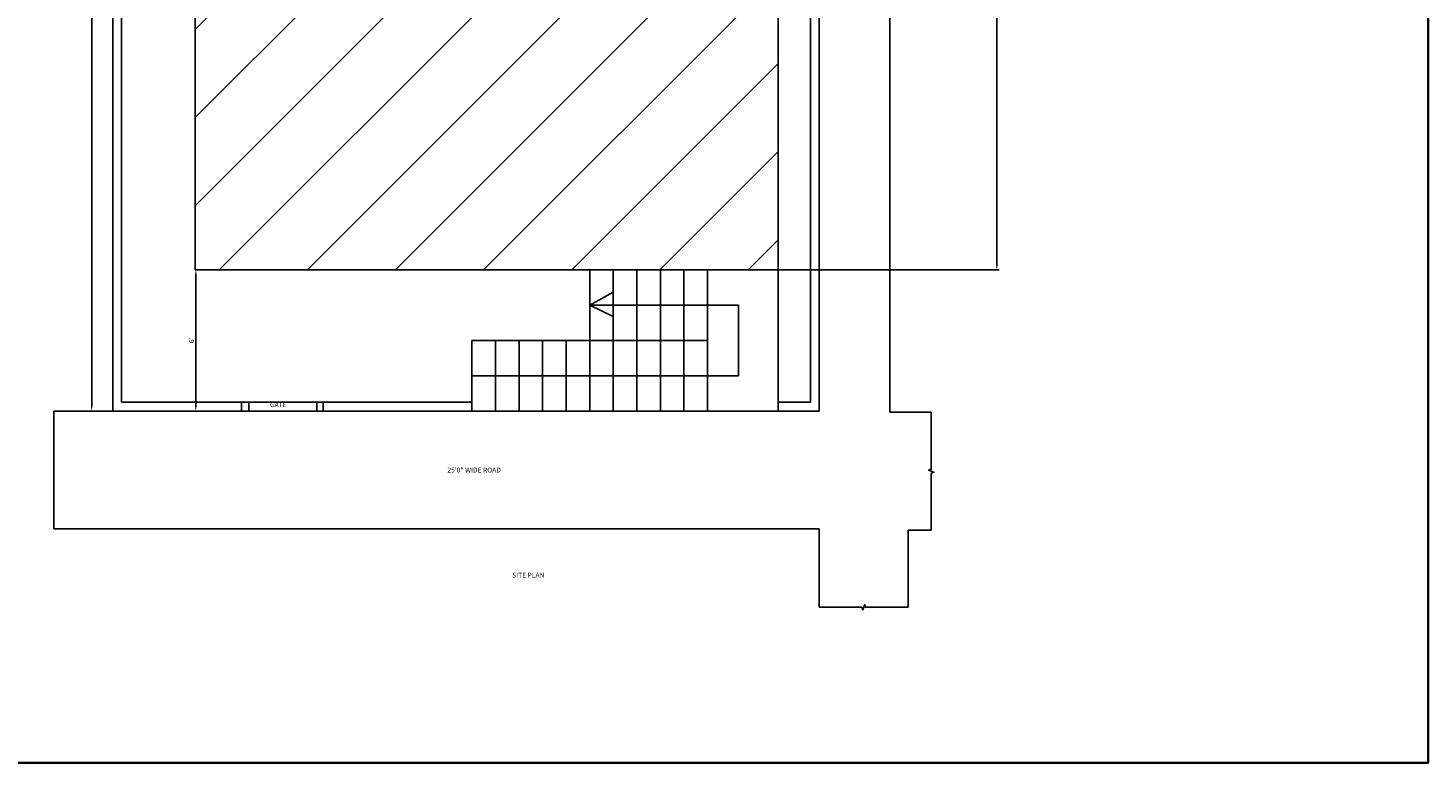
# Model space of a CAD drawing. Units: inches. Extents: x 2020 to 7901, y 1581 to 3943.
# Tile 12 of 17: x 3486 to 4199, y 1581 to 1955. Entities that reach past the tile are written whole.
import ezdxf

# ---------------------------------------------------------------- set-up
doc = ezdxf.new("R2010")
doc.units = ezdxf.units.IN
for name, color, linetype, lineweight in [('A-ANNO-DIMS', 2, 'Continuous', 18), ('A-ANNO-TEXT', 7, 'Continuous', 18), ('A-ANNO-TTLB', 7, 'Continuous', 35), ('A-FLOR-STRS', 3, 'Continuous', 25), ('C-PROP', 6, 'Continuous', 25), ('C-PROP-PATT', 8, 'Continuous', 13)]:
    doc.layers.add(name, color=color, linetype=linetype, lineweight=lineweight)
doc.styles.get("Standard").update_dxf_attribs({"font": 'arial.ttf'})
doc.dimstyles.new('ISO-25', dxfattribs={"dimtxt": 2.5, "dimasz": 2.5, "dimexe": 1.25, "dimexo": 0.625, "dimtad": 1, "dimdec": 1, "dimlunit": 3, "dimtxsty": 'Standard', "dimcen": 2.5, "dimadec": 0, "dimazin": 0, "dimtfac": 1, "dimtdec": 1, "dimtmove": 0, "dimatfit": 3, "dimfxl": 1, "dimarcsym": 0})

# ---------------------------------------------------------------- blocks, each defined once
blk = doc.blocks.new('*D11')
at = {"layer": 'A-ANNO-DIMS', "color": 0, "lineweight": -2, "transparency": 16777216}
for p, q in [((3571.28, 1829.56), (3571.28, 1762.56)), ((3571.55, 1832.06), (3572.53, 1832.06)), ((3571.55, 1760.06), (3572.53, 1760.06))]:
    blk.add_line(p, q, dxfattribs=at)
at = {"layer": 'A-ANNO-DIMS', "color": 0, "transparency": 16777216}
for points in [[(3570.86, 1829.56), (3571.7, 1829.56), (3571.28, 1832.06)], [(3570.86, 1762.56), (3571.7, 1762.56), (3571.28, 1760.06)]]:
    blk.add_solid(points, dxfattribs=at)
at = {"layer": 'DEFPOINTS', "color": 0, "transparency": 16777216}
for p in [(3570.93, 1832.06), (3570.93, 1760.06), (3571.28, 1760.06)]:
    blk.add_point(p, dxfattribs=at)
at = {"layer": 'A-ANNO-DIMS', "color": 0, "transparency": 16777216, "insert": (3569.38, 1796.06), "char_height": 2.5, "attachment_point": 5, "rotation": 90}
blk.add_mtext("6'", dxfattribs=at)
blk = doc.blocks.new('*D16')
at = {"layer": 'A-ANNO-DIMS', "color": 0, "lineweight": -2, "transparency": 16777216}
for p, q in [((3528.3, 2240.06), (3517, 2240.06)), ((3518.25, 2237.56), (3518.25, 1762.56)), ((3528.3, 1760.06), (3517, 1760.06))]:
    blk.add_line(p, q, dxfattribs=at)
at = {"layer": 'A-ANNO-DIMS', "color": 0, "transparency": 16777216}
for points in [[(3517.83, 2237.56), (3518.67, 2237.56), (3518.25, 2240.06)], [(3517.83, 1762.56), (3518.67, 1762.56), (3518.25, 1760.06)]]:
    blk.add_solid(points, dxfattribs=at)
at = {"layer": 'DEFPOINTS', "color": 0, "transparency": 16777216}
for p in [(3528.93, 2240.06), (3518.25, 1760.06), (3528.93, 1760.06)]:
    blk.add_point(p, dxfattribs=at)
at = {"layer": 'A-ANNO-DIMS', "color": 0, "transparency": 16777216, "insert": (3516.35, 2000.06), "char_height": 2.5, "attachment_point": 5, "rotation": 90}
blk.add_mtext("40'", dxfattribs=at)
blk = doc.blocks.new('*D61')
at = {"layer": 'A-ANNO-DIMS', "color": 0, "lineweight": -2, "transparency": 16777216}
for p, q in [((3868.55, 2214.06), (3980.6, 2214.06)), ((3979.35, 2211.56), (3979.35, 1834.56)), ((3868.55, 1832.06), (3980.6, 1832.06))]:
    blk.add_line(p, q, dxfattribs=at)
at = {"layer": 'A-ANNO-DIMS', "color": 0, "transparency": 16777216}
for points in [[(3978.93, 2211.56), (3979.77, 2211.56), (3979.35, 2214.06)], [(3978.93, 1834.56), (3979.77, 1834.56), (3979.35, 1832.06)]]:
    blk.add_solid(points, dxfattribs=at)
at = {"layer": 'DEFPOINTS', "color": 0, "transparency": 16777216}
for p in [(3867.93, 2214.06), (3867.93, 1832.06), (3979.35, 1832.06)]:
    blk.add_point(p, dxfattribs=at)
at = {"layer": 'A-ANNO-DIMS', "color": 0, "transparency": 16777216, "insert": (3977.45, 2023.06), "char_height": 2.5, "attachment_point": 5, "rotation": 90}
blk.add_mtext('31\'-10"', dxfattribs=at)

msp = doc.modelspace()

# ---------------------------------------------------------------- hatches: boundary and pattern name
at = {"layer": 'C-PROP-PATT'}
h = msp.add_hatch(dxfattribs=at)
h.set_pattern_fill('ANSI31', color=256, scale=10)
h.paths.add_polyline_path([(3867.93, 2214.06), (3570.93, 2214.06), (3570.93, 1832.06), (3867.93, 1832.06)])
h.paths.add_polyline_path([(3709.57, 2034.94), (3730.23, 2034.94), (3730.23, 2044.3), (3709.57, 2044.3)], flags=24)

# ---------------------------------------------------------------- linework, layer by layer
at = {"layer": 'A-ANNO-TTLB'}
msp.add_lwpolyline([(2019.8, 3067.25), (4199.03, 3067.25), (4199.03, 1580.73), (2019.8, 1580.73)], close=True, dxfattribs=at)
at = {"layer": 'A-FLOR-STRS'}
for p, q in [((3771.93, 1832.06), (3771.93, 1760.06)), ((3783.93, 1832.06), (3783.93, 1760.06)), ((3795.93, 1832.06), (3795.93, 1760.06)), ((3807.93, 1832.06), (3807.93, 1760.06)), ((3819.93, 1832.06), (3819.93, 1760.06)), ((3831.93, 1832.06), (3831.93, 1760.06)), ((3771.93, 1814.06), (3783.93, 1820.62)), ((3847.78, 1814.06), (3771.93, 1814.06)), ((3771.93, 1814.06), (3783.93, 1808.21)), ((3847.78, 1778.06), (3847.78, 1814.06)), ((3711.93, 1796.06), (3711.93, 1760.06)), ((3831.93, 1796.06), (3711.93, 1796.06)), ((3723.93, 1796.06), (3723.93, 1760.06)), ((3735.93, 1796.06), (3735.93, 1760.06)), ((3747.93, 1796.06), (3747.93, 1760.06)), ((3759.93, 1796.06), (3759.93, 1760.06)), ((3711.93, 1778.06), (3847.78, 1778.06))]:
    msp.add_line(p, q, dxfattribs=at)
at = {"layer": 'C-PROP'}
for p, q in [((3924.93, 2277.91), (3924.93, 1759.48)), ((3528.93, 1760.06), (3528.93, 2240.06)), ((3888.93, 2240.06), (3888.93, 1760.06)), ((3533.43, 1764.56), (3533.43, 2235.56)), ((3884.43, 2235.56), (3884.43, 1764.56)), ((3570.93, 1832.06), (3570.93, 2214.06)), ((3867.93, 2214.06), (3867.93, 1832.06)), ((3867.93, 1832.06), (3570.93, 1832.06)), ((3867.93, 1832.06), (3867.93, 1760.06)), ((3711.93, 1764.56), (3533.43, 1764.56)), ((3594.55, 1764.56), (3594.55, 1760.06)), ((3598.25, 1764.56), (3598.25, 1760.06)), ((3632.86, 1764.56), (3632.86, 1760.06)), ((3636.13, 1764.56), (3636.13, 1760.06)), ((3884.43, 1764.56), (3867.93, 1764.56)), ((3528.93, 1760.06), (3499.02, 1760.06)), ((3499.02, 1760.06), (3499.02, 1700.06)), ((3888.93, 1760.06), (3528.93, 1760.06)), ((3945.98, 1759.48), (3924.93, 1759.48)), ((3499.02, 1700.06), (3888.93, 1700.06)), ((3888.93, 1700.06), (3888.93, 1660.06)), ((3945.98, 1699.28), (3934.13, 1699.28)), ((3934.13, 1699.28), (3934.13, 1660.06))]:
    msp.add_line(p, q, dxfattribs=at)
for points in [[(3945.98, 1759.48), (3945.98, 1730.38), (3944.6, 1729.88), (3947.35, 1728.88), (3945.98, 1728.38), (3945.98, 1699.28)], [(3888.93, 1660.06), (3910.53, 1660.06), (3911.03, 1658.69), (3912.03, 1661.43), (3912.53, 1660.06), (3934.13, 1660.06)]]:
    msp.add_lwpolyline(points, dxfattribs=at)

# ---------------------------------------------------------------- texts
at = {"layer": 'A-ANNO-TEXT', "char_height": 2.5, "attachment_point": 1}
for s, width, insert in [('GATE', 39.6302, (3609.06, 1764.56)), ('25\'0" WIDE ROAD', 172.8221, (3699.46, 1731.24)), ('SITE PLAN', 174.0973, (3732.46, 1677.71))]:
    msp.add_mtext_dynamic_manual_height_columns(s, width=width, gutter_width=12.5, heights=[0], dxfattribs=dict(at, insert=insert))

# ---------------------------------------------------------------- dimensions: what is measured, and where the dimension line sits
at = {"layer": 'A-ANNO-DIMS'}
for base, p1, p2, override, picture, middle in [((3518.25, 1760.06), (3528.93, 2240.06), (3528.93, 1760.06), {"dimclrd": 0, "dimclre": 0, "dimclrt": 0}, '*D16', (3516.35, 2000.06)), ((3979.35, 1832.06), (3867.93, 2214.06), (3867.93, 1832.06), {"dimdec": 1, "dimlfac": 1, "dimrnd": 0, "dimzin": 1, "dimdsep": 46, "dimlunit": 4, "dimfrac": 2}, '*D61', (3977.45, 2023.06)), ((3571.28, 1760.06), (3570.93, 1832.06), (3570.93, 1760.06), {"dimclrd": 0, "dimclre": 0, "dimclrt": 0}, '*D11', (3569.38, 1796.06))]:
    dim = msp.add_linear_dim(base=base, p1=p1, p2=p2, angle=90, dimstyle='ISO-25', override=override, dxfattribs=at)
    dim.commit()
    dim.dimension.update_dxf_attribs({"geometry": picture, "text_midpoint": middle})

doc.saveas('drawing.dxf')
